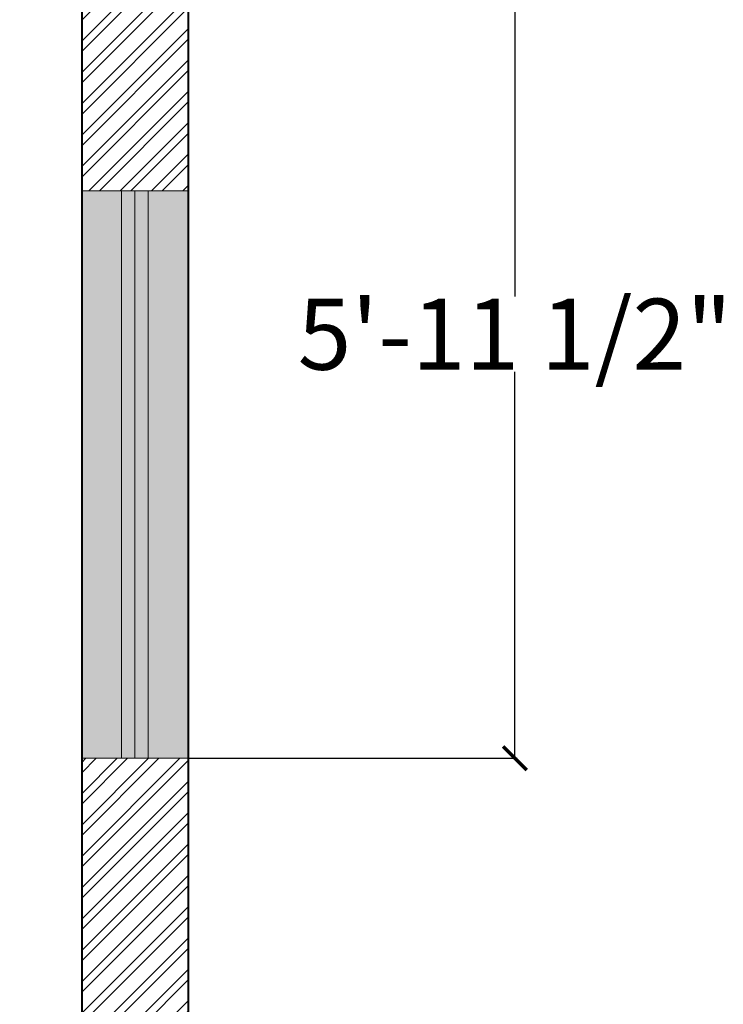
# Model space of a CAD drawing. Units: inches. Extents: x 528 to 2520, y -151 to 1354.
# Tile 40 of 41: x 2443 to 2502, y 731 to 815. Entities that reach past the tile are written whole.
import ezdxf

# ---------------------------------------------------------------- set-up
doc = ezdxf.new("R2010")
doc.units = ezdxf.units.IN
doc.header["$MEASUREMENT"] = 0
for name, color, linetype, lineweight in [('A-ANNO-DIMS', 2, 'Continuous', 18), ('A-ELEV-PROJ', 8, 'Continuous', 13), ('A-WALL-PATT', 6, 'Continuous', 13), ('walls', 7, 'Continuous', 40), ('WINDOWS', 2, 'Continuous', 20)]:
    doc.layers.add(name, color=color, linetype=linetype, lineweight=lineweight)
doc.layers.add('A-GLAZ-PATT', color=152, linetype='Continuous', lineweight=13, true_color=0x2776bb)
doc.styles.get("Standard").update_dxf_attribs({"font": 'arial.ttf'})
doc.dimstyles.get("Standard").update_dxf_attribs({"dimtxt": 6, "dimasz": 2, "dimexe": 0.18, "dimexo": 0.0625, "dimgap": 0.09, "dimtad": 0, "dimtih": 1, "dimtoh": 1, "dimdec": 1, "dimzin": 0, "dimdsep": 46, "dimlunit": 3, "dimtxsty": 'Standard', "dimblk": 'ARCHTICK', "dimcen": 0.09, "dimadec": 0, "dimazin": 0, "dimtfac": 1, "dimtdec": 1, "dimtofl": 0, "dimtmove": 0, "dimatfit": 3, "dimfxl": 1, "dimtolj": 1, "dimtzin": 0, "dimarcsym": 0})

# ---------------------------------------------------------------- blocks, each defined once
blk = doc.blocks.new('WINDOW-48x9-PLAN')
for p, q in [((0, 5.632), (48, 5.632)), ((0, 4.5), (48, 4.5)), ((0, 3.368), (48, 3.368))]:
    blk.add_line(p, q)
blk.add_lwpolyline([(0, 9), (48, 9), (48, 0), (0, 0)], close=True)
blk = doc.blocks.new('_ArchTick')
at = {"color": 0, "linetype": 'ByBlock', "const_width": 0.15}
blk.add_lwpolyline([(-0.5, -0.5), (0.5, 0.5)], dxfattribs=at)
blk = doc.blocks.new('*D98')
at = {"layer": 'A-ANNO-DIMS', "color": 0, "lineweight": -2, "transparency": 16777216}
for p, q in [((2448.075, 823.939), (2484.842, 823.939)), ((2484.662, 823.939), (2484.662, 791.264)), ((2484.662, 752.205), (2484.662, 784.879)), ((2457.075, 752.205), (2484.842, 752.205))]:
    blk.add_line(p, q, dxfattribs=at)
at = {"layer": 'Defpoints', "color": 0, "transparency": 16777216}
for p in [(2448.012, 823.939), (2484.662, 823.939), (2457.012, 752.205)]:
    blk.add_point(p, dxfattribs=at)
at = {"layer": 'A-ANNO-DIMS', "color": 0, "lineweight": -2, "transparency": 16777216, "xscale": 2, "yscale": 2, "zscale": 2}
for p, rotation in [((2484.662, 823.939), 90), ((2484.662, 752.205), 270)]:
    blk.add_blockref('_ArchTick', p, dxfattribs=dict(at, rotation=rotation))
at = {"layer": 'A-ANNO-DIMS', "color": 0, "transparency": 16777216, "insert": (2484.662, 788.072), "char_height": 6, "attachment_point": 5}
blk.add_mtext('\\A1;5\'-11 1/2"', dxfattribs=at)

msp = doc.modelspace()

# ---------------------------------------------------------------- hatches: boundary and pattern name
at = {"layer": 'A-GLAZ-PATT'}
h = msp.add_hatch(color=256, dxfattribs=at)
h.dxf.hatch_style = 1
h.paths.add_polyline_path([(2448.012, 800.205), (2448.012, 752.205), (2451.38, 752.205), (2451.38, 800.205)])
h.paths.add_polyline_path([(2451.38, 800.205), (2451.38, 752.205), (2452.512, 752.205), (2452.512, 800.205)])
h.paths.add_polyline_path([(2452.512, 800.205), (2452.512, 752.205), (2453.644, 752.205), (2453.644, 800.205)])
h.paths.add_polyline_path([(2453.644, 800.205), (2453.644, 752.205), (2457.012, 752.205), (2457.012, 800.205)])
at = {"layer": 'A-WALL-PATT'}
h = msp.add_hatch(dxfattribs=at)
h.set_pattern_fill('ANSI32', color=256, scale=5)
h.set_pattern_definition([(45, (1571.3155, -419.1643), (-1.3258252, 1.3258252), []), (45, (1572.1993, -419.1643), (-1.3258252, 1.3258252), [])])
h.paths.add_polyline_path([(2167.012, 744.691), (2158.012, 744.691), (2158.012, 549.939), (2169.559, 549.939), (2174.559, 549.939), (2174.559, 554.939), (2167.012, 554.939), (2167.012, 662.939), (2263.012, 662.939), (2263.012, 667.939), (2263.012, 686.939), (2269.012, 686.939), (2269.012, 691.939), (2258.012, 691.939), (2258.012, 667.939), (2167.012, 667.939)])
h.paths.add_polyline_path([(2260.017, 554.939), (2222.559, 554.939), (2222.559, 549.939), (2260.017, 549.939)])
h.paths.add_polyline_path([(2457.012, 752.205), (2448.012, 752.205), (2448.012, 691.939), (2358.012, 691.939), (2358.012, 686.939), (2448.012, 686.939), (2448.012, 554.939), (2358.012, 554.939), (2358.012, 549.939), (2448.012, 549.939), (2448.012, 405.939), (2406.012, 405.939), (2406.012, 396.939), (2457.012, 396.939)])
h.paths.add_polyline_path([(2457.012, 897.939), (2447.968, 897.939), (2447.968, 888.939), (2448.012, 888.939), (2448.012, 828.939), (2394.012, 828.939), (2394.012, 823.939), (2448.012, 823.939), (2448.012, 800.205), (2457.012, 800.205)])
h.paths.add_polyline_path([(2423.968, 897.939), (2359.012, 897.939), (2359.012, 828.939), (2355.579, 828.939), (2355.579, 823.939), (2364.012, 823.939), (2364.012, 829.939), (2364.012, 888.939), (2423.968, 888.939)])
h.paths.add_polyline_path([(2256.012, 897.939), (2191.012, 897.939), (2191.012, 888.939), (2251.012, 888.939), (2251.012, 828.939), (2251.012, 823.939), (2256.012, 823.939), (2256.012, 829.084)])
h.paths.add_polyline_path([(2167.012, 888.939), (2167.012, 897.939), (2158.012, 897.939), (2158.012, 792.691), (2167.012, 792.691), (2167.012, 823.939), (2221.012, 823.939), (2221.012, 828.939), (2167.012, 828.939)])
h.paths.add_polyline_path([(2316.012, 549.939), (2316.012, 554.939), (2296.017, 554.939), (2296.017, 549.939), (2311.012, 549.939), (2311.012, 455.122), (2316.012, 455.122)])
h.paths.add_polyline_path([(2311.012, 549.939), (2299.012, 549.939), (2299.012, 545.953), (2302.051, 545.953), (2302.051, 542.512), (2305.75, 542.512), (2305.75, 538.075), (2311.012, 538.075)], flags=17)
h.paths.add_polyline_path([(2358.012, 405.939), (2316.012, 405.939), (2316.012, 413.122), (2311.012, 413.122), (2311.012, 396.939), (2358.012, 396.939)])

# ---------------------------------------------------------------- linework, layer by layer
at = {"layer": 'A-ELEV-PROJ'}
msp.add_line((2457.012, 360.939), (2457.012, 897.939), dxfattribs=at)
at = {"layer": 'walls'}
for p, q in [((2457.012, 897.939), (2457.012, 396.939)), ((2448.012, 823.939), (2448.012, 691.939))]:
    msp.add_line(p, q, dxfattribs=at)

# ---------------------------------------------------------------- block references
at = {"layer": 'WINDOWS', "rotation": 90.00000000000055}
msp.add_blockref('WINDOW-48x9-PLAN', (2457.012, 752.205), dxfattribs=at)

# ---------------------------------------------------------------- dimensions: what is measured, and where the dimension line sits
at = {"layer": 'A-ANNO-DIMS'}
dim = msp.add_linear_dim(base=(2484.662, 823.939), p1=(2457.012, 752.205), p2=(2448.012, 823.939), angle=90, dimstyle='Standard', override={"dimdec": 1, "dimlfac": 1, "dimrnd": 0, "dimzin": 1, "dimdsep": 46, "dimlunit": 4, "dimfrac": 2}, dxfattribs=at)
dim.commit()
dim.dimension.update_dxf_attribs({"geometry": '*D98', "text_midpoint": (2484.662, 788.072)})

doc.saveas('drawing.dxf')
